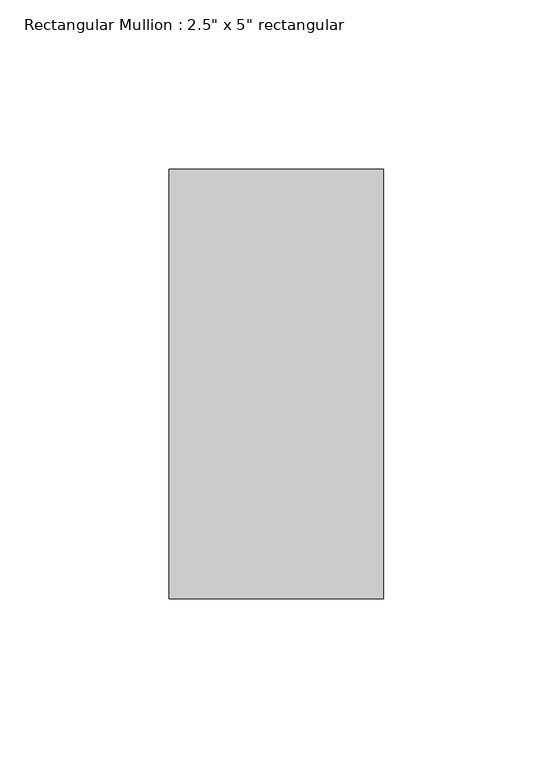
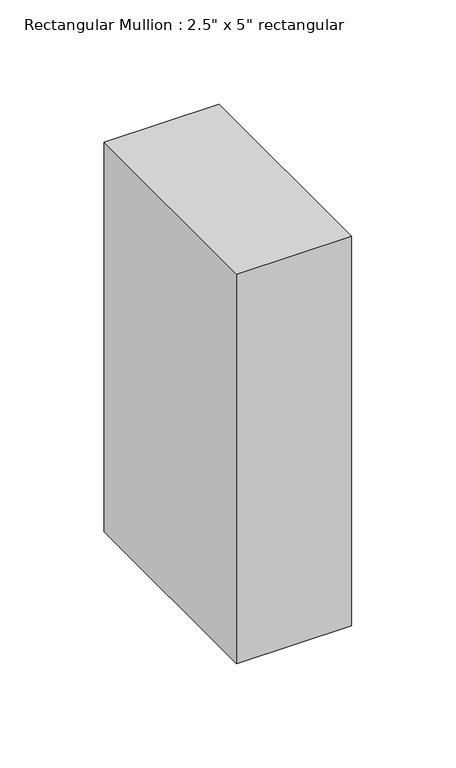
"""IFC4 building model written with IfcOpenShell, lengths in millimetres: member geometry."""

from ifc_helpers import new_model, si_unit, frame, origin, place, context, project, spatial, polyline, outline, extrude, source, transform, mapped, element, save


def member_bb91b9b7(model_context):
    return source(origin(), model_context, "Body", "SweptSolid", [
        extrude(outline(polyline([(0.0, 63.5), (0.0, -63.5), (-63.5, -63.5), (-63.5, 63.5), (0.0, 63.5)])), frame((0.0, 0.0, -227.8549185), z_axis=(0.0, 0.0, 1.0), x_axis=(1.0, 0.0, 0.0)), (0.0, 0.0, 1.0), 227.8549185),
    ])


if __name__ == "__main__":
    model = new_model("IFC4")
    model_context = context("Model", 3, world=origin())
    ifc_project = project(units=[si_unit("LENGTHUNIT", "METRE", prefix="MILLI")], contexts=[model_context])
    site = spatial("IfcSite", under=ifc_project)
    building = spatial("IfcBuilding", under=site)
    placement = place(None, origin())
    member_shape = member_bb91b9b7(model_context)
    element("IfcMember", 1, ObjectType="Rectangular Mullion : 2.5\" x 5\" rectangular", at=placement, inside=building, context=model_context, shape_type="MappedRepresentation", body=[
        mapped(member_shape, transform((0.0, 0.0, 0.0), x_axis=(1.0, 0.0, 0.0), y_axis=(0.0, 1.0, 0.0), z_axis=(0.0, 0.0, 1.0))),
    ])
    save(model, "model.ifc")

# Revit data of these elements
# Type "Rectangular Mullion : 2.5\" x 5\" rectangular"
#   built-in parameter 1007304 = 0.416667 (stored number, unit not read)
#   built-in parameter 1007301 = 0.104167 (stored number, unit not read)
#   built-in parameter 1007300 = 0.104167 (stored number, unit not read)
# Element 1 (IfcMember, "Rectangular Mullion : 2.5\" x 5\" rectangular")
#   Materials on its faces: "mullions"
# Materials
#   "mullions": class "Generic", colour RGB 120 120 120, transparency 0, Cost = 0
